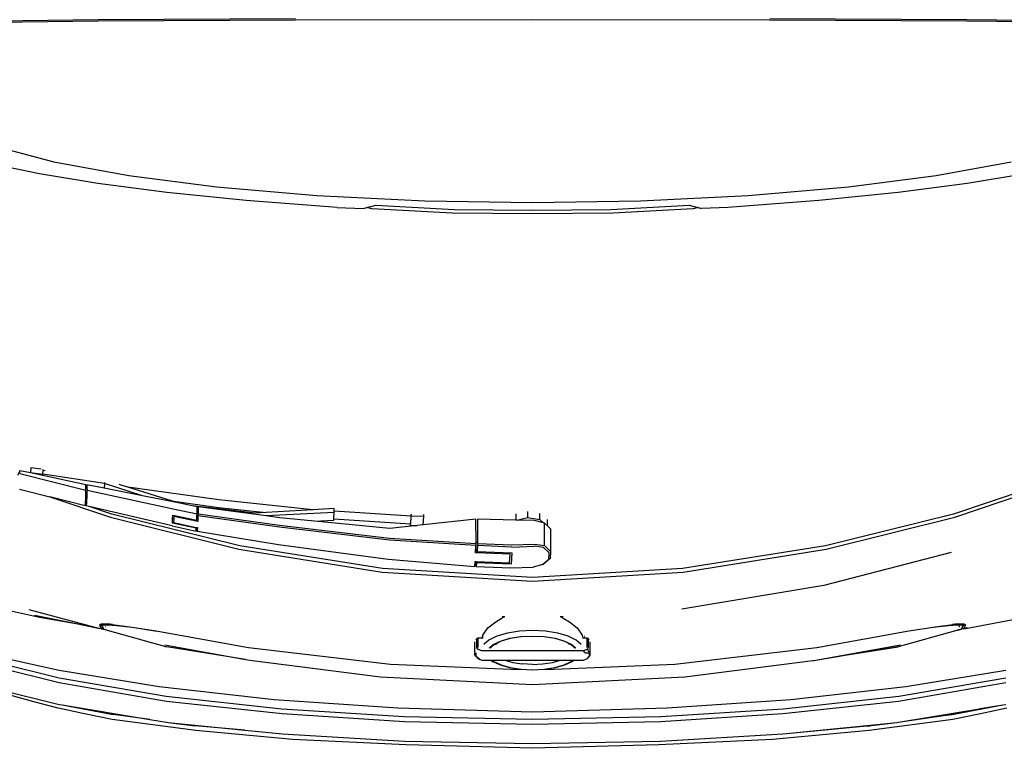
# Model space of a CAD drawing. Units: inches. Extents: x -4737294 to -4736756, y 1716389 to 1717040.
# Tile 4 of 25: x -4737168 to -4737133, y 1716465 to 1716491. Entities that reach past the tile are written whole.
import ezdxf

# ---------------------------------------------------------------- set-up
doc = ezdxf.new("R2010")
doc.units = ezdxf.units.IN
doc.header["$MEASUREMENT"] = 0
doc.layers.add('A-EQPM-VEHI', color=250, linetype='Continuous', lineweight=13)
doc.layers.add('Edges', color=250, linetype='Continuous')

# ---------------------------------------------------------------- blocks, each defined once
blk = doc.blocks.new('Nissan Qashqai pl')
at = {"layer": 'Edges'}
for p, q in [((11.06074, 12.39335), (11.05947, 12.28422)), ((11.06182, 12.39327), (11.06059, 12.28408)), ((11.47375, 12.27396), (11.44453, 12.36082)), ((11.44218, 12.3594), (11.47115, 12.27288)), ((11.18773, 12.33305), (11.19582, 12.2844)), ((11.56679, 12.28156), (11.55707, 12.33312)), ((11.18907, 12.25857), (11.17758, 12.32109)), ((11.6016, 12.31655), (11.61495, 12.23332)), ((11.6229, 12.22737), (11.60765, 12.31656)), ((11.61178, 12.31654), (11.62719, 12.22723)), ((11.63012, 12.31413), (11.62966, 12.31657)), ((11.63773, 12.27337), (11.63012, 12.31413)), ((11.63324, 12.29515), (11.63012, 12.31413)), ((11.63276, 12.31744), (11.63751, 12.29559)), ((11.63336, 12.29455), (11.63324, 12.29515)), ((11.63751, 12.29559), (11.64217, 12.27254)), ((11.64432, 12.22884), (11.63336, 12.29455)), ((11.05947, 12.28422), (11.0586, 12.11975)), ((11.06059, 12.28408), (11.05972, 12.11965)), ((11.19582, 12.2844), (11.2033, 12.22693)), ((11.56255, 12.27715), (11.56271, 12.28171)), ((11.56271, 12.28171), (11.56338, 12.28287)), ((11.56271, 12.28171), (11.56334, 12.28145)), ((11.56325, 12.2783), (11.56334, 12.28145)), ((11.56334, 12.28145), (11.56338, 12.28287)), ((11.56334, 12.28145), (11.56609, 12.2803)), ((11.56338, 12.28287), (11.56679, 12.28156)), ((11.56392, 12.28091), (11.56373, 12.27636)), ((11.56429, 12.28078), (11.56392, 12.28091)), ((11.56596, 12.28008), (11.56429, 12.28078)), ((11.56596, 12.28008), (11.56609, 12.2803)), ((11.56616, 12.27999), (11.56596, 12.28008)), ((11.56597, 12.28459), (11.56679, 12.28156)), ((11.56609, 12.2803), (11.56618, 12.27998)), ((11.56616, 12.27999), (11.56609, 12.2803)), ((11.56688, 12.27968), (11.56609, 12.2803)), ((11.56618, 12.27998), (11.56616, 12.27999)), ((11.56688, 12.27968), (11.56618, 12.27998)), ((11.56667, 12.28134), (11.56704, 12.27962)), ((11.56679, 12.28156), (11.56717, 12.27956)), ((11.56704, 12.27962), (11.56688, 12.27968)), ((11.56717, 12.27956), (11.56704, 12.27962)), ((11.56776, 12.27661), (11.56717, 12.27956)), ((11.47115, 12.27288), (11.49761, 12.16621)), ((11.50045, 12.16696), (11.47375, 12.27396)), ((11.50328, 12.27104), (11.53071, 12.16501)), ((11.56268, 12.2746), (11.56255, 12.27715)), ((11.56259, 12.27446), (11.56268, 12.2746)), ((11.5628, 12.2721), (11.56268, 12.2746)), ((11.56356, 12.27059), (11.56325, 12.2783)), ((11.56499, 12.25772), (11.56356, 12.27059)), ((11.56368, 12.27628), (11.56373, 12.27636)), ((11.56373, 12.27636), (11.56375, 12.27622)), ((11.56375, 12.27622), (11.56415, 12.2688)), ((11.56416, 12.27708), (11.56457, 12.27776)), ((11.56469, 12.27796), (11.56487, 12.27826)), ((11.5673, 12.27843), (11.56768, 12.27665)), ((11.56776, 12.27661), (11.58179, 12.22699)), ((11.56817, 12.27433), (11.56819, 12.27425)), ((11.5683, 12.27389), (11.56828, 12.27395)), ((11.56832, 12.27383), (11.56834, 12.27375)), ((11.63781, 12.27281), (11.63773, 12.27337)), ((11.63807, 12.27156), (11.63781, 12.27281)), ((11.63904, 12.26451), (11.63781, 12.27281)), ((11.63904, 12.26451), (11.63807, 12.27156)), ((11.64217, 12.27254), (11.65143, 12.20264)), ((11.56415, 12.2688), (11.56563, 12.25594)), ((11.64432, 12.22884), (11.63904, 12.26451)), ((11.19842, 12.18549), (11.18907, 12.25857)), ((11.56846, 12.23587), (11.56499, 12.25772)), ((11.58235, 12.15895), (11.56846, 12.23587)), ((11.61495, 12.23332), (11.62604, 12.13751)), ((11.2033, 12.22693), (11.20997, 12.16069)), ((11.59302, 12.15663), (11.57997, 12.22884)), ((11.58827, 12.18599), (11.58161, 12.22717)), ((11.58827, 12.18599), (11.58179, 12.22699)), ((11.63327, 12.131), (11.6229, 12.22737)), ((11.62719, 12.22723), (11.63768, 12.13077)), ((11.64462, 12.22707), (11.64432, 12.22884)), ((11.64478, 12.22577), (11.64462, 12.22707)), ((11.64738, 12.20422), (11.64478, 12.22577)), ((11.65393, 12.13376), (11.64478, 12.22577)), ((11.64741, 12.20385), (11.64738, 12.20422)), ((11.64749, 12.20324), (11.64741, 12.20385)), ((11.64795, 12.19805), (11.64749, 12.20324)), ((11.65393, 12.13376), (11.64795, 12.19805)), ((11.65143, 12.20264), (11.65888, 12.12224)), ((11.20565, 12.10185), (11.19842, 12.18549)), ((11.59302, 12.15663), (11.58827, 12.18599)), ((11.49761, 12.16621), (11.5166, 12.04708)), ((11.51964, 12.0475), (11.50045, 12.16696)), ((11.53071, 12.16501), (11.55039, 12.04664)), ((11.20997, 12.16069), (11.21586, 12.08501)), ((11.59629, 12.04057), (11.58235, 12.15895)), ((11.5932, 12.15564), (11.59302, 12.15663)), ((11.60675, 12.04892), (11.5932, 12.15564)), ((11.62604, 12.13751), (11.63292, 12.0344)), ((11.63993, 12.02899), (11.63327, 12.131)), ((11.63768, 12.13077), (11.64437, 12.02886)), ((11.65425, 12.1306), (11.65393, 12.13376)), ((11.66041, 12.02874), (11.65425, 12.1306)), ((11.05972, 12.11965), (11.05938, 11.92208)), ((11.65888, 12.12224), (11.66349, 12.02738)), ((11.21014, 12.01197), (11.20565, 12.10185)), ((11.21586, 12.08501), (11.21658, 12.06296)), ((11.2139, 12.05276), (11.21579, 12.05992)), ((11.21579, 12.05992), (11.21585, 12.06015)), ((11.21579, 12.05992), (11.21682, 12.056)), ((11.21585, 12.06015), (11.21658, 12.06296)), ((11.21585, 12.06015), (11.21682, 12.056)), ((11.21745, 11.98742), (11.2139, 12.05276)), ((11.21682, 12.056), (11.22044, 11.98904)), ((11.61327, 11.92208), (11.60675, 12.04892)), ((11.5166, 12.04708), (11.52386, 11.92208)), ((11.52698, 11.92208), (11.51964, 12.0475)), ((11.60051, 11.93346), (11.59629, 12.04057)), ((11.63292, 12.0344), (11.63628, 11.92208)), ((11.64211, 11.92208), (11.63993, 12.02899)), ((11.64437, 12.02886), (11.64655, 11.92208)), ((11.66226, 11.92208), (11.66041, 12.02874)), ((11.66349, 12.02738), (11.66628, 11.92208)), ((11.21164, 11.92208), (11.21014, 12.01197)), ((11.21801, 11.92208), (11.21745, 11.98742)), ((11.22044, 11.98904), (11.22108, 11.92208)), ((11.57479, 11.96843), (11.57457, 11.96768)), ((11.58239, 11.96768), (11.57457, 11.96768)), ((11.57457, 11.96768), (11.57457, 11.96395)), ((11.57617, 11.96938), (11.57479, 11.96843)), ((11.57479, 11.96843), (11.58262, 11.96843)), ((11.58846, 11.97008), (11.57758, 11.97008)), ((11.58262, 11.96843), (11.58377, 11.96782)), ((11.58668, 11.96947), (11.58377, 11.96782)), ((11.58377, 11.96782), (11.58513, 11.96453)), ((11.58679, 11.96604), (11.58668, 11.96947)), ((11.58961, 11.96947), (11.58668, 11.96947)), ((11.58846, 11.97008), (11.58961, 11.96947)), ((11.5915, 11.96782), (11.58961, 11.96947)), ((11.5915, 11.96782), (11.59043, 11.96839)), ((11.59285, 11.96453), (11.5915, 11.96782)), ((11.56082, 11.95281), (11.56588, 11.95938)), ((11.56588, 11.95938), (11.57195, 11.96347)), ((11.57195, 11.96347), (11.57457, 11.96395)), ((11.57261, 11.96533), (11.57261, 11.96561)), ((11.57613, 11.95845), (11.57286, 11.95178)), ((11.57306, 11.96528), (11.57306, 11.96569)), ((11.57457, 11.96395), (11.57457, 11.96378)), ((11.57994, 11.96265), (11.57613, 11.95845)), ((11.58679, 11.96604), (11.58513, 11.96453)), ((11.58513, 11.96453), (11.58513, 11.87963)), ((11.59285, 11.95694), (11.59285, 11.96453)), ((11.55816, 11.94815), (11.56082, 11.95281)), ((11.57286, 11.95178), (11.57035, 11.94308)), ((11.57692, 11.94885), (11.57987, 11.95487)), ((11.57876, 11.95169), (11.57712, 11.94834)), ((11.58001, 11.95424), (11.57876, 11.95169)), ((11.57876, 11.95169), (11.57995, 11.953)), ((11.57987, 11.95487), (11.58291, 11.95821)), ((11.58291, 11.95743), (11.58001, 11.95424)), ((11.59285, 11.95694), (11.59412, 11.95487)), ((11.59285, 11.95657), (11.59285, 11.95694)), ((11.59319, 11.9559), (11.59285, 11.95657)), ((11.59285, 11.95626), (11.59285, 11.95657)), ((11.59285, 11.95626), (11.59319, 11.9559)), ((11.59285, 11.95549), (11.59285, 11.95626)), ((11.59398, 11.95424), (11.59285, 11.95549)), ((11.59285, 11.94526), (11.59285, 11.95549)), ((11.59319, 11.9559), (11.59412, 11.95487)), ((11.59688, 11.94834), (11.59398, 11.95424)), ((11.59412, 11.95487), (11.59707, 11.94885)), ((11.55654, 11.94509), (11.55639, 11.94749)), ((11.55654, 11.94509), (11.55816, 11.94815)), ((11.57035, 11.94308), (11.56877, 11.93295)), ((11.57466, 11.94101), (11.57692, 11.94885)), ((11.57712, 11.94834), (11.5749, 11.94065)), ((11.59285, 11.8989), (11.59285, 11.94526)), ((11.59478, 11.93858), (11.59285, 11.94526)), ((11.5991, 11.94065), (11.59688, 11.94834)), ((11.59707, 11.94885), (11.59933, 11.94101)), ((11.48106, 11.93457), (11.47554, 11.93456)), ((11.48106, 11.93457), (11.4786, 11.93206)), ((11.48349, 11.93703), (11.48106, 11.93457)), ((11.48349, 11.93703), (11.50222, 11.93704)), ((11.49744, 11.93207), (11.50222, 11.93704)), ((11.50349, 11.93588), (11.49907, 11.93132)), ((11.50222, 11.93704), (11.50812, 11.93671)), ((11.50889, 11.93558), (11.50349, 11.93588)), ((11.50812, 11.93671), (11.51287, 11.9312)), ((11.50889, 11.93558), (11.51321, 11.93053)), ((11.57324, 11.93188), (11.57466, 11.94101)), ((11.5749, 11.94065), (11.5735, 11.93169)), ((11.59602, 11.93062), (11.59478, 11.93858)), ((11.60049, 11.93169), (11.5991, 11.94065)), ((11.59933, 11.94101), (11.60051, 11.93346)), ((11.47578, 11.92803), (11.47062, 11.92803)), ((11.47398, 11.91798), (11.47578, 11.92803)), ((11.47578, 11.92803), (11.4784, 11.93124)), ((11.4784, 11.93124), (11.47657, 11.92368)), ((11.4786, 11.93206), (11.4784, 11.93124)), ((11.49744, 11.93207), (11.4786, 11.93206)), ((11.49621, 11.92369), (11.49744, 11.93207)), ((11.49907, 11.93132), (11.49795, 11.92364)), ((11.51321, 11.93053), (11.51287, 11.9312)), ((11.51321, 11.93053), (11.51543, 11.92267)), ((11.56877, 11.93295), (11.56823, 11.92208)), ((11.57275, 11.92208), (11.57324, 11.93188)), ((11.5735, 11.93169), (11.57302, 11.92208)), ((11.59645, 11.92208), (11.59602, 11.93062)), ((11.60097, 11.92208), (11.60049, 11.93169)), ((11.60051, 11.93346), (11.60076, 11.93188)), ((11.60076, 11.93188), (11.60124, 11.92208)), ((11.05938, 11.92208), (11.05972, 11.72451)), ((11.21014, 11.8322), (11.21164, 11.92208)), ((11.21745, 11.85674), (11.21801, 11.92208)), ((11.22108, 11.92208), (11.22044, 11.85512)), ((11.46896, 11.91798), (11.47398, 11.91798)), ((11.47622, 11.90912), (11.47398, 11.91798)), ((11.47657, 11.92368), (11.47622, 11.90912)), ((11.49689, 11.90495), (11.49621, 11.92369)), ((11.49859, 11.9049), (11.49795, 11.92364)), ((11.51606, 11.90392), (11.51543, 11.92267)), ((11.52386, 11.92208), (11.5166, 11.79708)), ((11.51964, 11.79666), (11.52698, 11.92208)), ((11.56823, 11.92208), (11.56877, 11.91121)), ((11.57324, 11.91228), (11.57275, 11.92208)), ((11.57302, 11.92208), (11.5735, 11.91247)), ((11.59645, 11.92208), (11.59602, 11.91354)), ((11.60049, 11.91247), (11.60097, 11.92208)), ((11.60124, 11.92208), (11.60076, 11.91228)), ((11.60675, 11.79524), (11.61327, 11.92208)), ((11.63628, 11.92208), (11.63292, 11.80976)), ((11.63993, 11.81518), (11.64211, 11.92208)), ((11.64655, 11.92208), (11.64437, 11.8153)), ((11.66041, 11.81542), (11.66226, 11.92208)), ((11.66628, 11.92208), (11.66349, 11.81678)), ((11.56877, 11.91121), (11.57035, 11.90108)), ((11.57466, 11.90315), (11.57324, 11.91228)), ((11.5735, 11.91247), (11.5749, 11.90351)), ((11.59478, 11.90558), (11.59602, 11.91354)), ((11.59629, 11.80359), (11.60051, 11.91071)), ((11.5991, 11.90351), (11.60049, 11.91247)), ((11.60051, 11.91071), (11.59933, 11.90315)), ((11.60076, 11.91228), (11.60051, 11.91071)), ((11.47102, 11.90825), (11.4762, 11.90826)), ((11.4762, 11.90826), (11.47542, 11.87608)), ((11.47622, 11.90912), (11.4762, 11.90826)), ((11.49565, 11.87616), (11.49689, 11.90495)), ((11.49859, 11.9049), (11.49735, 11.87612)), ((11.50223, 11.8759), (11.50346, 11.90468)), ((11.50462, 11.90341), (11.50341, 11.87505)), ((11.50346, 11.90468), (11.51299, 11.90415)), ((11.51177, 11.90301), (11.50462, 11.90341)), ((11.51058, 11.87508), (11.51177, 11.90301)), ((11.51299, 11.90415), (11.51176, 11.87537)), ((11.51483, 11.87514), (11.51606, 11.90392)), ((11.57035, 11.90108), (11.57286, 11.89238)), ((11.57692, 11.89531), (11.57466, 11.90315)), ((11.5749, 11.90351), (11.57712, 11.89582)), ((11.59285, 11.8989), (11.59478, 11.90558)), ((11.59688, 11.89582), (11.5991, 11.90351)), ((11.59933, 11.90315), (11.59707, 11.89531)), ((11.55639, 11.89667), (11.55654, 11.89907)), ((11.55816, 11.89601), (11.55654, 11.89907)), ((11.56082, 11.89135), (11.55816, 11.89601)), ((11.57987, 11.88929), (11.57692, 11.89531)), ((11.57712, 11.89582), (11.57876, 11.89248)), ((11.59285, 11.88868), (11.59285, 11.8989)), ((11.59398, 11.88992), (11.59688, 11.89582)), ((11.59707, 11.89531), (11.59412, 11.88929)), ((11.56588, 11.88478), (11.56082, 11.89135)), ((11.57195, 11.88069), (11.56588, 11.88478)), ((11.57286, 11.89238), (11.57613, 11.88571)), ((11.57613, 11.88571), (11.57994, 11.88151)), ((11.57995, 11.89116), (11.57876, 11.89248)), ((11.57876, 11.89248), (11.58001, 11.88992)), ((11.58291, 11.88595), (11.57987, 11.88929)), ((11.58001, 11.88992), (11.58291, 11.88673)), ((11.59285, 11.88868), (11.59398, 11.88992)), ((11.59285, 11.88722), (11.59412, 11.88929)), ((11.59285, 11.8879), (11.59285, 11.88868)), ((11.59285, 11.88759), (11.59319, 11.88827)), ((11.59319, 11.88827), (11.59285, 11.8879)), ((11.59285, 11.88759), (11.59285, 11.8879)), ((11.59285, 11.88722), (11.59285, 11.88759)), ((11.59285, 11.87963), (11.59285, 11.88722)), ((11.59412, 11.88929), (11.59319, 11.88827)), ((11.57261, 11.88057), (11.57195, 11.88069)), ((11.57261, 11.88057), (11.57261, 11.88076)), ((11.57306, 11.88049), (11.57261, 11.88057)), ((11.57306, 11.88049), (11.57306, 11.88081)), ((11.57457, 11.88021), (11.57306, 11.88049)), ((11.57457, 11.88096), (11.57457, 11.88021)), ((11.57457, 11.88021), (11.57457, 11.87648)), ((11.57457, 11.87648), (11.58239, 11.87648)), ((11.57457, 11.87648), (11.57479, 11.87573)), ((11.58377, 11.87635), (11.58262, 11.87573)), ((11.58513, 11.87963), (11.58377, 11.87635)), ((11.58961, 11.87469), (11.5915, 11.87635)), ((11.59221, 11.87812), (11.59043, 11.87577)), ((11.59043, 11.87577), (11.5915, 11.87635)), ((11.5915, 11.87635), (11.59221, 11.87812)), ((11.59285, 11.87963), (11.59221, 11.87812)), ((11.49563, 11.87496), (11.47539, 11.87488)), ((11.47539, 11.87488), (11.4801, 11.83099)), ((11.47542, 11.87608), (11.49451, 11.87616)), ((11.49133, 11.80278), (11.49563, 11.87496)), ((11.49732, 11.87492), (11.49295, 11.80271)), ((11.49449, 11.87502), (11.49451, 11.87616)), ((11.50341, 11.87505), (11.49449, 11.87502)), ((11.49451, 11.87616), (11.49565, 11.87616)), ((11.49732, 11.87492), (11.49563, 11.87496)), ((11.49565, 11.87616), (11.49735, 11.87612)), ((11.50339, 11.87463), (11.49732, 11.87492)), ((11.49735, 11.87612), (11.50223, 11.8759)), ((11.50341, 11.87505), (11.50339, 11.87463)), ((11.50884, 11.80182), (11.5148, 11.87394)), ((11.51054, 11.87423), (11.51058, 11.87508)), ((11.5148, 11.87394), (11.51054, 11.87423)), ((11.51472, 11.8751), (11.51058, 11.87508)), ((11.51176, 11.87537), (11.51472, 11.87515)), ((11.51472, 11.87515), (11.51472, 11.8751)), ((11.51472, 11.87515), (11.51483, 11.87514)), ((11.51483, 11.87514), (11.51472, 11.8751)), ((11.58262, 11.87573), (11.57479, 11.87573)), ((11.57479, 11.87573), (11.57617, 11.87478)), ((11.58846, 11.87408), (11.57758, 11.87408)), ((11.58668, 11.87469), (11.58961, 11.87469)), ((11.58961, 11.87469), (11.58846, 11.87408)), ((11.59043, 11.87577), (11.58961, 11.87469)), ((11.2139, 11.7914), (11.21745, 11.85674)), ((11.22044, 11.85512), (11.21682, 11.78816)), ((11.20565, 11.74231), (11.21014, 11.8322)), ((11.47305, 11.83139), (11.47165, 11.83144)), ((11.47305, 11.83139), (11.473, 11.82087)), ((11.4801, 11.83099), (11.47305, 11.83139)), ((11.4801, 11.83099), (11.48065, 11.82584)), ((11.47281, 11.82086), (11.46872, 11.75675)), ((11.47111, 11.82093), (11.47189, 11.82089)), ((11.47281, 11.82086), (11.47189, 11.82089)), ((11.473, 11.82087), (11.47281, 11.82086)), ((11.47916, 11.8205), (11.473, 11.82087)), ((11.47508, 11.75641), (11.47919, 11.82046)), ((11.47919, 11.82046), (11.47916, 11.8205)), ((11.48062, 11.82044), (11.47919, 11.82046)), ((11.48062, 11.82044), (11.48065, 11.82584)), ((11.48065, 11.82584), (11.4831, 11.803)), ((11.63327, 11.71316), (11.63993, 11.81518)), ((11.64437, 11.8153), (11.63768, 11.7134)), ((11.65425, 11.71357), (11.66041, 11.81542)), ((11.66349, 11.81678), (11.65888, 11.72193)), ((11.4831, 11.803), (11.47707, 11.74042)), ((11.4805, 11.71128), (11.49133, 11.80278)), ((11.49295, 11.80271), (11.48212, 11.71121)), ((11.58235, 11.68521), (11.59629, 11.80359)), ((11.63292, 11.80976), (11.62604, 11.70665)), ((11.49642, 11.71041), (11.50884, 11.80182)), ((11.5166, 11.79708), (11.49761, 11.67796)), ((11.50045, 11.6772), (11.51964, 11.79666)), ((11.5932, 11.68852), (11.60675, 11.79524)), ((11.21579, 11.78424), (11.2139, 11.7914)), ((11.21682, 11.78816), (11.21579, 11.78424)), ((11.21682, 11.78816), (11.21585, 11.78401)), ((11.21585, 11.78401), (11.21579, 11.78424)), ((11.21658, 11.78121), (11.21585, 11.78401)), ((11.21586, 11.75915), (11.21658, 11.78121)), ((11.21586, 11.75915), (11.20997, 11.68347)), ((11.46872, 11.75675), (11.46649, 11.75682)), ((11.46649, 11.75682), (11.46757, 11.73891)), ((11.46975, 11.75671), (11.46872, 11.75675)), ((11.46975, 11.75671), (11.47273, 11.69994)), ((11.47508, 11.75641), (11.46975, 11.75671)), ((11.47611, 11.75636), (11.47508, 11.75641)), ((11.47707, 11.74042), (11.47611, 11.75636)), ((11.19842, 11.65867), (11.20565, 11.74231)), ((11.46757, 11.73891), (11.45941, 11.6607)), ((11.46757, 11.73891), (11.46992, 11.70014)), ((11.47707, 11.74042), (11.47428, 11.71144)), ((11.0586, 11.72441), (11.05947, 11.55994)), ((11.05972, 11.72451), (11.06059, 11.56009)), ((11.65888, 11.72193), (11.65143, 11.64152)), ((11.6229, 11.61679), (11.63327, 11.71316)), ((11.63768, 11.7134), (11.62719, 11.61693)), ((11.65114, 11.68233), (11.65425, 11.71357)), ((11.47094, 11.64327), (11.4805, 11.71128)), ((11.48212, 11.71121), (11.47257, 11.6432)), ((11.47428, 11.71144), (11.47273, 11.69994)), ((11.48539, 11.64249), (11.49642, 11.71041)), ((11.62604, 11.70665), (11.61495, 11.61084)), ((11.47273, 11.69994), (11.46512, 11.64343)), ((11.46576, 11.66035), (11.46992, 11.70014)), ((11.46992, 11.70014), (11.47047, 11.69095)), ((11.47047, 11.69095), (11.46419, 11.63849)), ((11.59218, 11.68277), (11.5932, 11.68852)), ((11.20997, 11.68347), (11.2033, 11.61723)), ((11.56846, 11.60829), (11.58235, 11.68521)), ((11.58021, 11.61555), (11.59218, 11.68277)), ((11.59218, 11.68277), (11.58179, 11.61717)), ((11.64478, 11.61839), (11.65114, 11.68233)), ((11.65114, 11.68233), (11.64749, 11.64092)), ((11.49761, 11.67796), (11.47115, 11.57128)), ((11.47375, 11.5702), (11.50045, 11.6772)), ((11.18907, 11.58559), (11.19842, 11.65867)), ((11.45941, 11.6607), (11.44866, 11.58459)), ((11.46024, 11.62121), (11.46576, 11.66035)), ((11.46419, 11.63849), (11.46114, 11.62406)), ((11.46505, 11.64255), (11.46419, 11.63849)), ((11.46792, 11.64248), (11.46505, 11.64255)), ((11.46512, 11.64343), (11.46801, 11.64335)), ((11.46687, 11.62247), (11.47088, 11.64239)), ((11.46801, 11.64335), (11.46792, 11.64248)), ((11.47088, 11.64239), (11.46792, 11.64248)), ((11.46801, 11.64335), (11.47094, 11.64327)), ((11.47252, 11.64233), (11.47088, 11.64239)), ((11.47094, 11.64327), (11.47257, 11.6432)), ((11.47212, 11.62223), (11.47625, 11.64214)), ((11.47439, 11.64223), (11.47252, 11.64233)), ((11.47257, 11.6432), (11.47449, 11.6431)), ((11.47727, 11.64296), (11.47315, 11.62305)), ((11.47439, 11.64223), (11.47449, 11.6431)), ((11.47625, 11.64214), (11.47439, 11.64223)), ((11.47449, 11.6431), (11.47727, 11.64296)), ((11.47827, 11.62277), (11.48226, 11.64167)), ((11.48298, 11.64165), (11.47879, 11.62186)), ((11.48098, 11.62171), (11.48532, 11.64161)), ((11.48226, 11.64167), (11.48244, 11.64254)), ((11.48226, 11.64167), (11.48298, 11.64165)), ((11.48244, 11.64254), (11.48247, 11.64267)), ((11.48535, 11.64246), (11.48244, 11.64254)), ((11.48247, 11.64267), (11.48535, 11.64246)), ((11.483, 11.64176), (11.48298, 11.64165)), ((11.48532, 11.64161), (11.483, 11.64176)), ((11.48539, 11.64249), (11.48535, 11.64246)), ((11.65143, 11.64152), (11.64217, 11.57162)), ((11.64478, 11.61839), (11.64749, 11.64092)), ((11.45125, 11.55073), (11.46687, 11.62247)), ((11.46083, 11.62261), (11.45585, 11.5969)), ((11.46114, 11.62406), (11.46024, 11.62121)), ((11.46114, 11.62406), (11.46083, 11.62261)), ((11.47495, 11.62207), (11.47212, 11.62223)), ((11.47315, 11.62305), (11.47515, 11.62294)), ((11.47495, 11.62207), (11.47515, 11.62294)), ((11.47879, 11.62186), (11.47495, 11.62207)), ((11.47515, 11.62294), (11.47827, 11.62277)), ((11.2033, 11.61723), (11.19582, 11.55976)), ((11.46024, 11.62121), (11.44866, 11.58459)), ((11.48098, 11.62171), (11.4649, 11.55261)), ((11.56776, 11.56755), (11.58179, 11.61717)), ((11.60765, 11.5276), (11.6229, 11.61679)), ((11.62719, 11.61693), (11.61178, 11.52762)), ((11.64227, 11.603), (11.64462, 11.61709)), ((11.64462, 11.61709), (11.64478, 11.61839)), ((11.56499, 11.58644), (11.56846, 11.60829)), ((11.56905, 11.60888), (11.56563, 11.58822)), ((11.61495, 11.61084), (11.6016, 11.52761)), ((11.63012, 11.53004), (11.64227, 11.603)), ((11.64227, 11.603), (11.63807, 11.5726)), ((11.45585, 11.5969), (11.44582, 11.56516)), ((11.45585, 11.5969), (11.44965, 11.56495)), ((11.17758, 11.52307), (11.18907, 11.58559)), ((11.44866, 11.58459), (11.44723, 11.58007)), ((11.56356, 11.57357), (11.56499, 11.58644)), ((11.56563, 11.58822), (11.56415, 11.57536)), ((11.44723, 11.58007), (11.44639, 11.57739)), ((11.56335, 11.56843), (11.56356, 11.57357)), ((11.56415, 11.57536), (11.56375, 11.56794)), ((11.44575, 11.56516), (11.43801, 11.51398)), ((11.4448, 11.5652), (11.44575, 11.56516)), ((11.44575, 11.56516), (11.44582, 11.56516)), ((11.44582, 11.56516), (11.44965, 11.56495)), ((11.44965, 11.56495), (11.44685, 11.5505)), ((11.45676, 11.51971), (11.47375, 11.5702)), ((11.47115, 11.57128), (11.4649, 11.55261)), ((11.56255, 11.56701), (11.56268, 11.56956)), ((11.56271, 11.56245), (11.56255, 11.56701)), ((11.56268, 11.56956), (11.56259, 11.5697)), ((11.56268, 11.56956), (11.5628, 11.57206)), ((11.56335, 11.56843), (11.56268, 11.56956)), ((11.56325, 11.56586), (11.56335, 11.56843)), ((11.56334, 11.56271), (11.56325, 11.56586)), ((11.56368, 11.56788), (11.56335, 11.56843)), ((11.56375, 11.56794), (11.56392, 11.56325)), ((11.56487, 11.5659), (11.56469, 11.5662)), ((11.56661, 11.56253), (11.56704, 11.56455)), ((11.56665, 11.56424), (11.56688, 11.56448)), ((11.56669, 11.5644), (11.56688, 11.56448)), ((11.56671, 11.56257), (11.56712, 11.56458)), ((11.56717, 11.5646), (11.56679, 11.56261)), ((11.56688, 11.56448), (11.56704, 11.56455)), ((11.56704, 11.56455), (11.56739, 11.56625)), ((11.56704, 11.56455), (11.56712, 11.56458)), ((11.56712, 11.56458), (11.56763, 11.56708)), ((11.56712, 11.56458), (11.56717, 11.5646)), ((11.56717, 11.5646), (11.56763, 11.56708)), ((11.56745, 11.56646), (11.56739, 11.56625)), ((11.56763, 11.56708), (11.56776, 11.56755)), ((11.63012, 11.53004), (11.63807, 11.5726)), ((11.64217, 11.57162), (11.63751, 11.54857)), ((11.05947, 11.55994), (11.06074, 11.45082)), ((11.06059, 11.56009), (11.06182, 11.4509)), ((11.19582, 11.55976), (11.18773, 11.51111)), ((11.55053, 11.5023), (11.56648, 11.56144)), ((11.56334, 11.56271), (11.56271, 11.56245)), ((11.56338, 11.56129), (11.56271, 11.56245)), ((11.56273, 11.5431), (11.56648, 11.56144)), ((11.56609, 11.56386), (11.56334, 11.56271)), ((11.56338, 11.56129), (11.56334, 11.56271)), ((11.56583, 11.56223), (11.56338, 11.56129)), ((11.56392, 11.56325), (11.56429, 11.56338)), ((11.56429, 11.56338), (11.56596, 11.56408)), ((11.56609, 11.56386), (11.56583, 11.56223)), ((11.56616, 11.56236), (11.56583, 11.56223)), ((11.56596, 11.56408), (11.56616, 11.56417)), ((11.56609, 11.56386), (11.56596, 11.56408)), ((11.56613, 11.56388), (11.56609, 11.56386)), ((11.56618, 11.56418), (11.56613, 11.56388)), ((11.56613, 11.56388), (11.56616, 11.56417)), ((11.56613, 11.56388), (11.56645, 11.5641)), ((11.56665, 11.56424), (11.56616, 11.56236)), ((11.56616, 11.56417), (11.56618, 11.56418)), ((11.56616, 11.56236), (11.56645, 11.5641)), ((11.56661, 11.56253), (11.56616, 11.56236)), ((11.56618, 11.56418), (11.56648, 11.56431)), ((11.56645, 11.5641), (11.56648, 11.56431)), ((11.56645, 11.5641), (11.56665, 11.56424)), ((11.56648, 11.56431), (11.56669, 11.5644)), ((11.56679, 11.56261), (11.56648, 11.56144)), ((11.56671, 11.56257), (11.56661, 11.56253)), ((11.56669, 11.5644), (11.56665, 11.56424)), ((11.56679, 11.56261), (11.56671, 11.56257)), ((11.43747, 11.49463), (11.45125, 11.54985)), ((11.44684, 11.54963), (11.43914, 11.51392)), ((11.44983, 11.54978), (11.44684, 11.54963)), ((11.44685, 11.5505), (11.44997, 11.55066)), ((11.44983, 11.54978), (11.44997, 11.55066)), ((11.45125, 11.54985), (11.44983, 11.54978)), ((11.44997, 11.55066), (11.45125, 11.55073)), ((11.45125, 11.55073), (11.4529, 11.55066)), ((11.4529, 11.54978), (11.45125, 11.54985)), ((11.4529, 11.55066), (11.45711, 11.55045)), ((11.45711, 11.54958), (11.4529, 11.54978)), ((11.46429, 11.54915), (11.45676, 11.51971)), ((11.45711, 11.55045), (11.45994, 11.5503)), ((11.46197, 11.5493), (11.45711, 11.54958)), ((11.45983, 11.54978), (11.45994, 11.5503)), ((11.46402, 11.54999), (11.45983, 11.54978)), ((11.45994, 11.5503), (11.46197, 11.55018)), ((11.46197, 11.55018), (11.46404, 11.55004)), ((11.46375, 11.54918), (11.46197, 11.5493)), ((11.46402, 11.54999), (11.46375, 11.54918)), ((11.46429, 11.54915), (11.46375, 11.54918)), ((11.46404, 11.55004), (11.46402, 11.54999)), ((11.46423, 11.55), (11.46402, 11.54999)), ((11.46404, 11.55004), (11.46423, 11.55)), ((11.46423, 11.55), (11.46424, 11.55003)), ((11.4643, 11.55002), (11.46423, 11.55)), ((11.4649, 11.55261), (11.4643, 11.55002)), ((11.63751, 11.54857), (11.63276, 11.52672)), ((11.55533, 11.50682), (11.56273, 11.5431)), ((11.55707, 11.51104), (11.56273, 11.5431)), ((11.6016, 11.52761), (11.58664, 11.46068)), ((11.58843, 11.44985), (11.60765, 11.5276)), ((11.61178, 11.52762), (11.59225, 11.44945)), ((11.61272, 11.45895), (11.62966, 11.52759)), ((11.63276, 11.52672), (11.62771, 11.50627)), ((11.62966, 11.52759), (11.63012, 11.53004)), ((11.16395, 11.47112), (11.17758, 11.52307)), ((11.43501, 11.51584), (11.43475, 11.51409)), ((11.45032, 11.49453), (11.45676, 11.51971)), ((11.18773, 11.51111), (11.17906, 11.46956)), ((11.43371, 11.51238), (11.43251, 11.50378)), ((11.43475, 11.51409), (11.43403, 11.51411)), ((11.43801, 11.51398), (11.43475, 11.51409)), ((11.4382, 11.51397), (11.43676, 11.50364)), ((11.43914, 11.51392), (11.43692, 11.50363)), ((11.4382, 11.51397), (11.43801, 11.51398)), ((11.43914, 11.51392), (11.4382, 11.51397)), ((11.54814, 11.47101), (11.55707, 11.51104)), ((11.43251, 11.50378), (11.43676, 11.50364)), ((11.43251, 11.50378), (11.4369, 11.50353)), ((11.4369, 11.50353), (11.435, 11.49469)), ((11.43676, 11.50364), (11.43692, 11.50363)), ((11.43692, 11.50363), (11.4369, 11.50353)), ((11.62771, 11.50627), (11.62241, 11.48743)), ((11.435, 11.49469), (11.43896, 11.49272)), ((11.43747, 11.49463), (11.435, 11.49469))]:
    blk.add_line(p, q, dxfattribs=at)
blk = doc.blocks.new('car')
blk.add_blockref('Nissan Qashqai pl', (-9.74328, -11.91512))

msp = doc.modelspace()

# ---------------------------------------------------------------- block references
at = {"layer": 'A-EQPM-VEHI', "xscale": 43.56002006885659, "yscale": 43.56002006885659, "zscale": 43.56002006885659, "rotation": 270}
msp.add_blockref('car', (-4737150.017, 1716548.61), dxfattribs=at)

doc.saveas('drawing.dxf')
